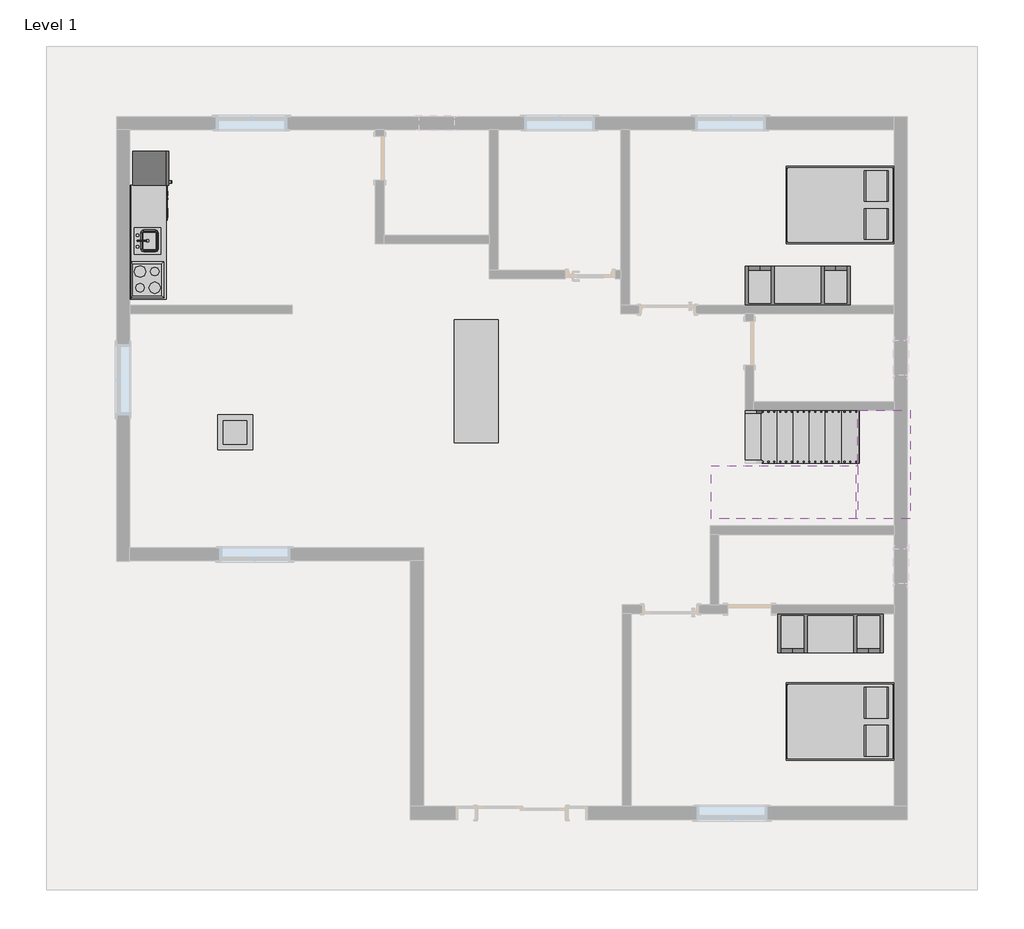
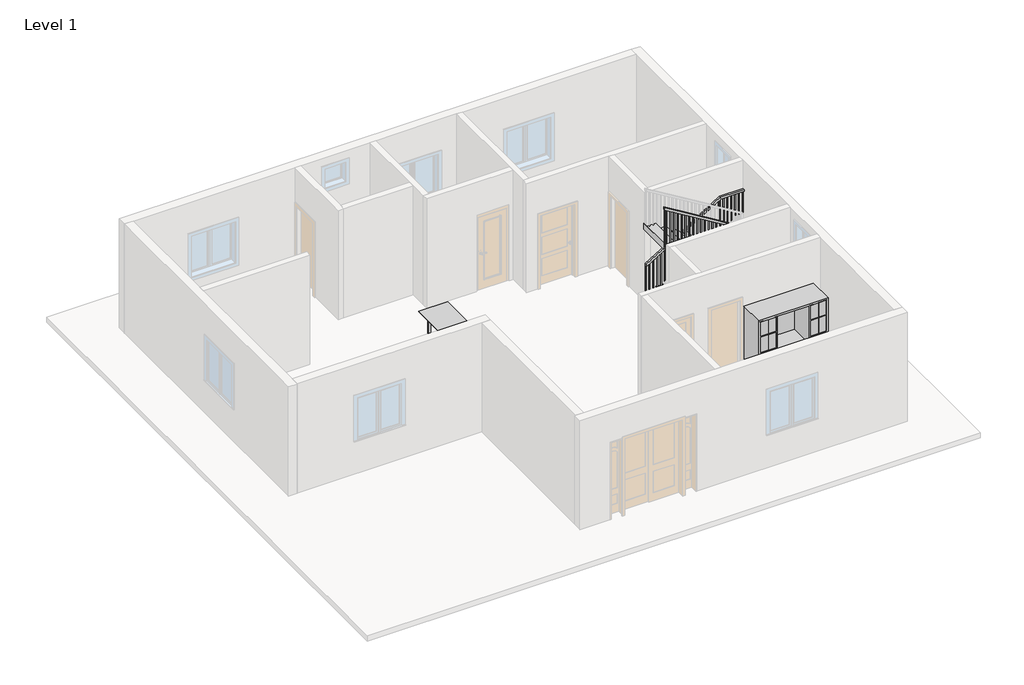
# One storey, part 2 of 2: 7 furniture elements, 4 proxies, 2 stair flights, 1 flow terminal, 1 railing, 1 slab.
"""IFC4 building model written with IfcOpenShell, lengths in millimetres."""

from ifc_helpers import new_model, si_unit, frame, origin, place, context, project, spatial, polyline, outline, extrude, faceted_brep, transform, mapped, element, save
from components import proxy_a6faaae8, proxy_45b28599, kitchenette_medium_0001_kitchenette_medium_0001_844211aa, proxy_c523a7b7, flow_terminal_871c2e40, furniture_c8abb964, furniture_c6510c7c, furniture_cf0b6580, furniture_b5c51a22, furniture_92191dda, non_monolithic_landing_284a18c3, stair_flight_c73b5a8b, stair_flight_e67f926d

model = new_model("IFC4")

# Units and contexts
model_context = context("Model", 3, world=origin())
ifc_project = project(units=[si_unit("LENGTHUNIT", "METRE", prefix="MILLI")], contexts=[model_context])

# Site, building, storey
site = spatial("IfcSite", under=ifc_project)
building = spatial("IfcBuilding", under=site)
storey = spatial("IfcBuildingStorey", under=building, Name="Level 1", Elevation=0.0)

# Proxies
placement = place(None, origin())
proxy_shape = proxy_a6faaae8(model_context)
element("IfcBuildingElementProxy", 1, Name="Cook Top-4 Unit2 : 22\" x 20\"", ObjectType="Cook Top-4 Unit2 : 22\" x 20\"", at=placement, inside=storey, context=model_context, shape_type="MappedRepresentation", body=[
    mapped(proxy_shape, transform((-14025.3866603, -262.6331121, 0.0), x_axis=(0.0, 1.0000000000000002, 0.0), y_axis=(-1.0000000000000002, 0.0, 0.0), z_axis=(0.0, 0.0, 1.0))),
])
proxy_2_shape = proxy_45b28599(model_context)
element("IfcBuildingElementProxy", 2, Name="Dishwasher : 24\" x 24\" x 34\"", ObjectType="Dishwasher : 24\" x 24\" x 34\"", at=placement, inside=storey, context=model_context, shape_type="MappedRepresentation", body=[
    mapped(proxy_2_shape, transform((-13733.5370955, 688.5494195, 0.0), x_axis=(0.0, 1.0000000000000002, 0.0), y_axis=(-1.0000000000000002, 0.0, 0.0), z_axis=(0.0, 0.0, 1.0))),
])
kitchenette_medium_0001_kitchenette_medium_0001_shape = kitchenette_medium_0001_kitchenette_medium_0001_844211aa(model_context)
element("IfcBuildingElementProxy", 3, Name="Kitchenette - Medium.0001 : Kitchenette - Medium.0001", ObjectType="Kitchenette - Medium.0001 : Kitchenette - Medium.0001", at=placement, inside=storey, context=model_context, shape_type="MappedRepresentation", body=[
    mapped(kitchenette_medium_0001_kitchenette_medium_0001_shape, transform((-14330.1866603, 61.529183, 0.0), x_axis=(0.0, 1.0000000000000002, 0.0), y_axis=(-1.0000000000000002, 0.0, 0.0), z_axis=(0.0, 0.0, 1.0))),
])
proxy_3_shape = proxy_c523a7b7(model_context)
element("IfcBuildingElementProxy", 4, Name="Refrigerator : 24\" x 25\" LH", ObjectType="Refrigerator : 24\" x 25\" LH", at=placement, inside=storey, context=model_context, shape_type="MappedRepresentation", body=[
    mapped(proxy_3_shape, transform((-13979.7376888, 1674.1168879, 0.0), x_axis=(0.0, 1.0000000000000002, 0.0), y_axis=(-1.0000000000000002, 0.0, 0.0), z_axis=(0.0, 0.0, 1.0))),
])

# Flow terminal
flow_terminal_shape = flow_terminal_871c2e40(model_context)
element("IfcFlowTerminal", 5, ObjectType="Sink Kitchen-Island : 18\" x 18\"", at=placement, inside=storey, context=model_context, shape_type="MappedRepresentation", body=[
    mapped(flow_terminal_shape, transform((-14023.0412592, 394.7776474, -14.4), x_axis=(0.0, 1.0000000000000002, 0.0), y_axis=(-1.0000000000000002, 0.0, 0.0), z_axis=(0.0, 0.0, 1.0))),
])

# Furniture
furniture_shape = furniture_c8abb964(model_context)
element("IfcFurniture", 6, ObjectType="Bed-Box : Double 53\" x 74\"", at=placement, inside=storey, context=model_context, shape_type="MappedRepresentation", body=[
    mapped(furniture_shape, transform((-1751.3571521, 1371.919347, 0.0), x_axis=(0.0, -0.9999999999999998, 0.0), y_axis=(0.9999999999999998, 0.0, 0.0), z_axis=(0.0, 0.0, 1.0))),
])
element("IfcFurniture", 7, ObjectType="Bed-Box : Double 53\" x 74\"", at=placement, inside=storey, context=model_context, shape_type="MappedRepresentation", body=[
    mapped(furniture_shape, transform((-1751.3571521, -7606.980653, 0.0), x_axis=(0.0, -1.0, 0.0), y_axis=(1.0, 0.0, 0.0), z_axis=(0.0, 0.0, 1.0))),
])
furniture_2_shape = furniture_c6510c7c(model_context)
element("IfcFurniture", 8, ObjectType="Counter Top w Sink Hole : 24\" Depth", at=placement, inside=storey, context=model_context, shape_type="MappedRepresentation", body=[
    mapped(furniture_2_shape, transform((-14330.1866603, 594.929183, -14.4), x_axis=(0.0, 1.0000000000000002, 0.0), y_axis=(-1.0000000000000002, 0.0, 0.0), z_axis=(0.0, 0.0, 1.0))),
])
furniture_3_shape = furniture_cf0b6580(model_context)
element("IfcFurniture", 9, ObjectType="Entertainment Center : 72\" x 72\" x 24\"", at=placement, inside=storey, context=model_context, shape_type="MappedRepresentation", body=[
    mapped(furniture_3_shape, transform((-2722.3866603, -808.7331121, 0.0), x_axis=(-1.0, 0.0, 0.0), y_axis=(0.0, -1.0, 0.0), z_axis=(0.0, 0.0, 1.0))),
])
element("IfcFurniture", 10, ObjectType="Entertainment Center : 72\" x 72\" x 24\"", at=placement, inside=storey, context=model_context, shape_type="MappedRepresentation", body=[
    mapped(furniture_3_shape, transform((-2150.8866603, -5964.9331121, 0.0), x_axis=(1.0000000000000002, 0.0, 0.0), y_axis=(0.0, 1.0000000000000002, 0.0), z_axis=(0.0, 0.0, 1.0))),
])
furniture_4_shape = furniture_b5c51a22(model_context)
element("IfcFurniture", 11, ObjectType="Table-Coffee : 24\" x 24\" x 24\"", at=placement, inside=storey, context=model_context, shape_type="MappedRepresentation", body=[
    mapped(furniture_4_shape, transform((-12519.6524269, -3012.1441899, 0.0), x_axis=(1.0, 0.0, 0.0), y_axis=(0.0, 1.0, 0.0), z_axis=(0.0, 0.0, 1.0))),
])
furniture_5_shape = furniture_92191dda(model_context)
element("IfcFurniture", 12, ObjectType="Table-Dining : 30\" x 84\" x 22\"", at=placement, inside=storey, context=model_context, shape_type="MappedRepresentation", body=[
    mapped(furniture_5_shape, transform((-8215.1755825, -2046.1988787, 0.0), x_axis=(0.0, 1.0, 0.0), y_axis=(-1.0, 0.0, 0.0), z_axis=(0.0, 0.0, 1.0))),
])

# Railing
element("IfcRailing", 13, ObjectType="Handrail - Rectangular", at=placement, inside=storey, context=model_context, shape_type="SolidModel", body=[
    faceted_brep([(-3636.7866603, -2535.9331121, 1083.7333333), (-3636.7866603, -2535.9331121, 1024.3318731), (-3636.7866603, -2586.7331121, 1024.3318731), (-3636.7866603, -2586.7331121, 1083.7333333), (-1680.9866603, -2535.9331121, 2269.0666667), (-1666.7942508, -2535.9331121, 2218.2666667), (-1666.7942508, -2586.7331121, 2218.2666667), (-1680.9866603, -2586.7331121, 2269.0666667), (-766.5866603, -2535.9331121, 2269.0666667), (-766.5866603, -2535.9331121, 2218.2666667), (-817.3866603, -2586.7331121, 2218.2666667), (-817.3866603, -2586.7331121, 2269.0666667), (-766.5866603, -4415.5331121, 2269.0666667), (-766.5866603, -4415.5331121, 2218.2666667), (-817.3866603, -4364.7331121, 2218.2666667), (-817.3866603, -4364.7331121, 2269.0666667), (-1401.5866603, -4415.5331121, 2269.0666667), (-1415.7790697, -4415.5331121, 2218.2666667), (-1415.7790697, -4364.7331121, 2218.2666667), (-1401.5866603, -4364.7331121, 2269.0666667), (-4195.5866603, -4415.5331121, 3962.4), (-4195.5866603, -4364.7331121, 3962.4), (-4195.5866603, -4364.7331121, 3902.9985397), (-4195.5866603, -4415.5331121, 3902.9985397)], [[[0, 1, 2, 3]], [[1, 0, 4, 5]], [[2, 1, 5, 6]], [[3, 2, 6, 7]], [[0, 3, 7, 4]], [[5, 4, 8, 9]], [[6, 5, 9, 10]], [[7, 6, 10, 11]], [[4, 7, 11, 8]], [[9, 8, 12, 13]], [[10, 9, 13, 14]], [[11, 10, 14, 15]], [[8, 11, 15, 12]], [[13, 12, 16, 17]], [[14, 13, 17, 18]], [[15, 14, 18, 19]], [[12, 15, 19, 16]], [[20, 21, 22, 23]], [[17, 16, 20, 23]], [[18, 17, 23, 22]], [[19, 18, 22, 21]], [[16, 19, 21, 20]]]),
    extrude(outline(polyline([(3877.9833882, -4154.3116603), (2878.6666667, -4154.3116603), (2878.6666667, -4135.2616603), (3866.4379337, -4135.2616603), (3877.9833882, -4154.3116603)])), frame((0.0, -4399.6581121, 0.0), z_axis=(0.0, 1.0, 0.0), x_axis=(0.0, 0.0, 1.0)), (0.0, 0.0, 1.0), 19.05),
    extrude(outline(polyline([(3816.4076307, -4052.7116603), (2878.6666667, -4052.7116603), (2878.6666667, -4033.6616603), (3804.8621761, -4033.6616603), (3816.4076307, -4052.7116603)])), frame((0.0, -4399.6581121, 0.0), z_axis=(0.0, 1.0, 0.0), x_axis=(0.0, 0.0, 1.0)), (0.0, 0.0, 1.0), 19.05),
    extrude(outline(polyline([(3754.8318731, -3951.1116603), (2878.6666667, -3951.1116603), (2878.6666667, -3932.0616603), (3743.2864185, -3932.0616603), (3754.8318731, -3951.1116603)])), frame((0.0, -4399.6581121, 0.0), z_axis=(0.0, 1.0, 0.0), x_axis=(0.0, 0.0, 1.0)), (0.0, 0.0, 1.0), 19.05),
    extrude(outline(polyline([(3693.2561155, -3849.5116603), (2709.3333333, -3849.5116603), (2709.3333333, -3830.4616603), (3681.710661, -3830.4616603), (3693.2561155, -3849.5116603)])), frame((0.0, -4399.6581121, 0.0), z_axis=(0.0, 1.0, 0.0), x_axis=(0.0, 0.0, 1.0)), (0.0, 0.0, 1.0), 19.05),
    extrude(outline(polyline([(3631.6803579, -3747.9116603), (2709.3333333, -3747.9116603), (2709.3333333, -3728.8616603), (3620.1349034, -3728.8616603), (3631.6803579, -3747.9116603)])), frame((0.0, -4399.6581121, 0.0), z_axis=(0.0, 1.0, 0.0), x_axis=(0.0, 0.0, 1.0)), (0.0, 0.0, 1.0), 19.05),
    extrude(outline(polyline([(3570.1046004, -3646.3116603), (2709.3333333, -3646.3116603), (2709.3333333, -3627.2616603), (3558.5591458, -3627.2616603), (3570.1046004, -3646.3116603)])), frame((0.0, -4399.6581121, 0.0), z_axis=(0.0, 1.0, 0.0), x_axis=(0.0, 0.0, 1.0)), (0.0, 0.0, 1.0), 19.05),
    extrude(outline(polyline([(3508.5288428, -3544.7116603), (2540.0, -3544.7116603), (2540.0, -3525.6616603), (3496.9833882, -3525.6616603), (3508.5288428, -3544.7116603)])), frame((0.0, -4399.6581121, 0.0), z_axis=(0.0, 1.0, 0.0), x_axis=(0.0, 0.0, 1.0)), (0.0, 0.0, 1.0), 19.05),
    extrude(outline(polyline([(3446.9530852, -3443.1116603), (2540.0, -3443.1116603), (2540.0, -3424.0616603), (3435.4076307, -3424.0616603), (3446.9530852, -3443.1116603)])), frame((0.0, -4399.6581121, 0.0), z_axis=(0.0, 1.0, 0.0), x_axis=(0.0, 0.0, 1.0)), (0.0, 0.0, 1.0), 19.05),
    extrude(outline(polyline([(3385.3773276, -3341.5116603), (2370.6666667, -3341.5116603), (2370.6666667, -3322.4616603), (3373.8318731, -3322.4616603), (3385.3773276, -3341.5116603)])), frame((0.0, -4399.6581121, 0.0), z_axis=(0.0, 1.0, 0.0), x_axis=(0.0, 0.0, 1.0)), (0.0, 0.0, 1.0), 19.05),
    extrude(outline(polyline([(3323.80157, -3239.9116603), (2370.6666667, -3239.9116603), (2370.6666667, -3220.8616603), (3312.2561155, -3220.8616603), (3323.80157, -3239.9116603)])), frame((0.0, -4399.6581121, 0.0), z_axis=(0.0, 1.0, 0.0), x_axis=(0.0, 0.0, 1.0)), (0.0, 0.0, 1.0), 19.05),
    extrude(outline(polyline([(3262.2258125, -3138.3116603), (2370.6666667, -3138.3116603), (2370.6666667, -3119.2616603), (3250.6803579, -3119.2616603), (3262.2258125, -3138.3116603)])), frame((0.0, -4399.6581121, 0.0), z_axis=(0.0, 1.0, 0.0), x_axis=(0.0, 0.0, 1.0)), (0.0, 0.0, 1.0), 19.05),
    extrude(outline(polyline([(3200.6500549, -3036.7116603), (2201.3333333, -3036.7116603), (2201.3333333, -3017.6616603), (3189.1046004, -3017.6616603), (3200.6500549, -3036.7116603)])), frame((0.0, -4399.6581121, 0.0), z_axis=(0.0, 1.0, 0.0), x_axis=(0.0, 0.0, 1.0)), (0.0, 0.0, 1.0), 19.05),
    extrude(outline(polyline([(3139.0742973, -2935.1116603), (2201.3333333, -2935.1116603), (2201.3333333, -2916.0616603), (3127.5288428, -2916.0616603), (3139.0742973, -2935.1116603)])), frame((0.0, -4399.6581121, 0.0), z_axis=(0.0, 1.0, 0.0), x_axis=(0.0, 0.0, 1.0)), (0.0, 0.0, 1.0), 19.05),
    extrude(outline(polyline([(3077.4985397, -2833.5116603), (2201.3333333, -2833.5116603), (2201.3333333, -2814.4616603), (3065.9530852, -2814.4616603), (3077.4985397, -2833.5116603)])), frame((0.0, -4399.6581121, 0.0), z_axis=(0.0, 1.0, 0.0), x_axis=(0.0, 0.0, 1.0)), (0.0, 0.0, 1.0), 19.05),
    extrude(outline(polyline([(3015.9227822, -2731.9116603), (2032.0, -2731.9116603), (2032.0, -2712.8616603), (3004.3773276, -2712.8616603), (3015.9227822, -2731.9116603)])), frame((0.0, -4399.6581121, 0.0), z_axis=(0.0, 1.0, 0.0), x_axis=(0.0, 0.0, 1.0)), (0.0, 0.0, 1.0), 19.05),
    extrude(outline(polyline([(2954.3470246, -2630.3116603), (2032.0, -2630.3116603), (2032.0, -2611.2616603), (2942.80157, -2611.2616603), (2954.3470246, -2630.3116603)])), frame((0.0, -4399.6581121, 0.0), z_axis=(0.0, 1.0, 0.0), x_axis=(0.0, 0.0, 1.0)), (0.0, 0.0, 1.0), 19.05),
    extrude(outline(polyline([(2892.771267, -2528.7116603), (2032.0, -2528.7116603), (2032.0, -2509.6616603), (2881.2258125, -2509.6616603), (2892.771267, -2528.7116603)])), frame((0.0, -4399.6581121, 0.0), z_axis=(0.0, 1.0, 0.0), x_axis=(0.0, 0.0, 1.0)), (0.0, 0.0, 1.0), 19.05),
    extrude(outline(polyline([(2831.1955094, -2427.1116603), (1862.6666667, -2427.1116603), (1862.6666667, -2408.0616603), (2819.6500549, -2408.0616603), (2831.1955094, -2427.1116603)])), frame((0.0, -4399.6581121, 0.0), z_axis=(0.0, 1.0, 0.0), x_axis=(0.0, 0.0, 1.0)), (0.0, 0.0, 1.0), 19.05),
    extrude(outline(polyline([(2769.6197519, -2325.5116603), (1862.6666667, -2325.5116603), (1862.6666667, -2306.4616603), (2758.0742973, -2306.4616603), (2769.6197519, -2325.5116603)])), frame((0.0, -4399.6581121, 0.0), z_axis=(0.0, 1.0, 0.0), x_axis=(0.0, 0.0, 1.0)), (0.0, 0.0, 1.0), 19.05),
    extrude(outline(polyline([(2708.0439943, -2223.9116603), (1693.3333333, -2223.9116603), (1693.3333333, -2204.8616603), (2696.4985397, -2204.8616603), (2708.0439943, -2223.9116603)])), frame((0.0, -4399.6581121, 0.0), z_axis=(0.0, 1.0, 0.0), x_axis=(0.0, 0.0, 1.0)), (0.0, 0.0, 1.0), 19.05),
    extrude(outline(polyline([(2646.4682367, -2122.3116603), (1693.3333333, -2122.3116603), (1693.3333333, -2103.2616603), (2634.9227822, -2103.2616603), (2646.4682367, -2122.3116603)])), frame((0.0, -4399.6581121, 0.0), z_axis=(0.0, 1.0, 0.0), x_axis=(0.0, 0.0, 1.0)), (0.0, 0.0, 1.0), 19.05),
    extrude(outline(polyline([(2584.8924791, -2020.7116603), (1693.3333333, -2020.7116603), (1693.3333333, -2001.6616603), (2573.3470246, -2001.6616603), (2584.8924791, -2020.7116603)])), frame((0.0, -4399.6581121, 0.0), z_axis=(0.0, 1.0, 0.0), x_axis=(0.0, 0.0, 1.0)), (0.0, 0.0, 1.0), 19.05),
    extrude(outline(polyline([(2523.3167216, -1919.1116603), (1524.0, -1919.1116603), (1524.0, -1900.0616603), (2511.771267, -1900.0616603), (2523.3167216, -1919.1116603)])), frame((0.0, -4399.6581121, 0.0), z_axis=(0.0, 1.0, 0.0), x_axis=(0.0, 0.0, 1.0)), (0.0, 0.0, 1.0), 19.05),
    extrude(outline(polyline([(2461.740964, -1817.5116603), (1524.0, -1817.5116603), (1524.0, -1798.4616603), (2450.1955094, -1798.4616603), (2461.740964, -1817.5116603)])), frame((0.0, -4399.6581121, 0.0), z_axis=(0.0, 1.0, 0.0), x_axis=(0.0, 0.0, 1.0)), (0.0, 0.0, 1.0), 19.05),
    extrude(outline(polyline([(2400.1652064, -1715.9116603), (1524.0, -1715.9116603), (1524.0, -1696.8616603), (2388.6197519, -1696.8616603), (2400.1652064, -1715.9116603)])), frame((0.0, -4399.6581121, 0.0), z_axis=(0.0, 1.0, 0.0), x_axis=(0.0, 0.0, 1.0)), (0.0, 0.0, 1.0), 19.05),
    extrude(outline(polyline([(2338.5894488, -1614.3116603), (1354.6666667, -1614.3116603), (1354.6666667, -1595.2616603), (2327.0439943, -1595.2616603), (2338.5894488, -1614.3116603)])), frame((0.0, -4399.6581121, 0.0), z_axis=(0.0, 1.0, 0.0), x_axis=(0.0, 0.0, 1.0)), (0.0, 0.0, 1.0), 19.05),
    extrude(outline(polyline([(2277.0136913, -1512.7116603), (1354.6666667, -1512.7116603), (1354.6666667, -1493.6616603), (2265.4682367, -1493.6616603), (2277.0136913, -1512.7116603)])), frame((0.0, -4399.6581121, 0.0), z_axis=(0.0, 1.0, 0.0), x_axis=(0.0, 0.0, 1.0)), (0.0, 0.0, 1.0), 19.05),
    extrude(outline(polyline([(-1290.4616603, -4399.6581121), (-1309.5116603, -4399.6581121), (-1309.5116603, -4380.6081121), (-1290.4616603, -4380.6081121), (-1290.4616603, -4399.6581121)])), frame((0.0, 0.0, 1354.6666667), z_axis=(0.0, 0.0, 1.0), x_axis=(1.0, 0.0, 0.0)), (0.0, 0.0, 1.0), 863.6),
    extrude(outline(polyline([(-1188.8616603, -4399.6581121), (-1207.9116603, -4399.6581121), (-1207.9116603, -4380.6081121), (-1188.8616603, -4380.6081121), (-1188.8616603, -4399.6581121)])), frame((0.0, 0.0, 1354.6666667), z_axis=(0.0, 0.0, 1.0), x_axis=(1.0, 0.0, 0.0)), (0.0, 0.0, 1.0), 863.6),
    extrude(outline(polyline([(-1087.2616603, -4399.6581121), (-1106.3116603, -4399.6581121), (-1106.3116603, -4380.6081121), (-1087.2616603, -4380.6081121), (-1087.2616603, -4399.6581121)])), frame((0.0, 0.0, 1354.6666667), z_axis=(0.0, 0.0, 1.0), x_axis=(1.0, 0.0, 0.0)), (0.0, 0.0, 1.0), 863.6),
    extrude(outline(polyline([(-985.6616603, -4399.6581121), (-1004.7116603, -4399.6581121), (-1004.7116603, -4380.6081121), (-985.6616603, -4380.6081121), (-985.6616603, -4399.6581121)])), frame((0.0, 0.0, 1354.6666667), z_axis=(0.0, 0.0, 1.0), x_axis=(1.0, 0.0, 0.0)), (0.0, 0.0, 1.0), 863.6),
    extrude(outline(polyline([(-884.0616603, -4399.6581121), (-903.1116603, -4399.6581121), (-903.1116603, -4380.6081121), (-884.0616603, -4380.6081121), (-884.0616603, -4399.6581121)])), frame((0.0, 0.0, 1354.6666667), z_axis=(0.0, 0.0, 1.0), x_axis=(1.0, 0.0, 0.0)), (0.0, 0.0, 1.0), 863.6),
    extrude(outline(polyline([(-782.4616603, -4279.0081121), (-782.4616603, -4298.0581121), (-801.5116603, -4298.0581121), (-801.5116603, -4279.0081121), (-782.4616603, -4279.0081121)])), frame((0.0, 0.0, 1354.6666667), z_axis=(0.0, 0.0, 1.0), x_axis=(1.0, 0.0, 0.0)), (0.0, 0.0, 1.0), 863.6),
    extrude(outline(polyline([(-782.4616603, -4177.4081121), (-782.4616603, -4196.4581121), (-801.5116603, -4196.4581121), (-801.5116603, -4177.4081121), (-782.4616603, -4177.4081121)])), frame((0.0, 0.0, 1354.6666667), z_axis=(0.0, 0.0, 1.0), x_axis=(1.0, 0.0, 0.0)), (0.0, 0.0, 1.0), 863.6),
    extrude(outline(polyline([(-782.4616603, -4075.8081121), (-782.4616603, -4094.8581121), (-801.5116603, -4094.8581121), (-801.5116603, -4075.8081121), (-782.4616603, -4075.8081121)])), frame((0.0, 0.0, 1354.6666667), z_axis=(0.0, 0.0, 1.0), x_axis=(1.0, 0.0, 0.0)), (0.0, 0.0, 1.0), 863.6),
    extrude(outline(polyline([(-782.4616603, -3974.2081121), (-782.4616603, -3993.2581121), (-801.5116603, -3993.2581121), (-801.5116603, -3974.2081121), (-782.4616603, -3974.2081121)])), frame((0.0, 0.0, 1354.6666667), z_axis=(0.0, 0.0, 1.0), x_axis=(1.0, 0.0, 0.0)), (0.0, 0.0, 1.0), 863.6),
    extrude(outline(polyline([(-782.4616603, -3872.6081121), (-782.4616603, -3891.6581121), (-801.5116603, -3891.6581121), (-801.5116603, -3872.6081121), (-782.4616603, -3872.6081121)])), frame((0.0, 0.0, 1354.6666667), z_axis=(0.0, 0.0, 1.0), x_axis=(1.0, 0.0, 0.0)), (0.0, 0.0, 1.0), 863.6),
    extrude(outline(polyline([(-782.4616603, -3771.0081121), (-782.4616603, -3790.0581121), (-801.5116603, -3790.0581121), (-801.5116603, -3771.0081121), (-782.4616603, -3771.0081121)])), frame((0.0, 0.0, 1354.6666667), z_axis=(0.0, 0.0, 1.0), x_axis=(1.0, 0.0, 0.0)), (0.0, 0.0, 1.0), 863.6),
    extrude(outline(polyline([(-782.4616603, -3669.4081121), (-782.4616603, -3688.4581121), (-801.5116603, -3688.4581121), (-801.5116603, -3669.4081121), (-782.4616603, -3669.4081121)])), frame((0.0, 0.0, 1354.6666667), z_axis=(0.0, 0.0, 1.0), x_axis=(1.0, 0.0, 0.0)), (0.0, 0.0, 1.0), 863.6),
    extrude(outline(polyline([(-782.4616603, -3567.8081121), (-782.4616603, -3586.8581121), (-801.5116603, -3586.8581121), (-801.5116603, -3567.8081121), (-782.4616603, -3567.8081121)])), frame((0.0, 0.0, 1354.6666667), z_axis=(0.0, 0.0, 1.0), x_axis=(1.0, 0.0, 0.0)), (0.0, 0.0, 1.0), 863.6),
    extrude(outline(polyline([(-782.4616603, -3466.2081121), (-782.4616603, -3485.2581121), (-801.5116603, -3485.2581121), (-801.5116603, -3466.2081121), (-782.4616603, -3466.2081121)])), frame((0.0, 0.0, 1354.6666667), z_axis=(0.0, 0.0, 1.0), x_axis=(1.0, 0.0, 0.0)), (0.0, 0.0, 1.0), 863.6),
    extrude(outline(polyline([(-782.4616603, -3364.6081121), (-782.4616603, -3383.6581121), (-801.5116603, -3383.6581121), (-801.5116603, -3364.6081121), (-782.4616603, -3364.6081121)])), frame((0.0, 0.0, 1354.6666667), z_axis=(0.0, 0.0, 1.0), x_axis=(1.0, 0.0, 0.0)), (0.0, 0.0, 1.0), 863.6),
    extrude(outline(polyline([(-782.4616603, -3263.0081121), (-782.4616603, -3282.0581121), (-801.5116603, -3282.0581121), (-801.5116603, -3263.0081121), (-782.4616603, -3263.0081121)])), frame((0.0, 0.0, 1354.6666667), z_axis=(0.0, 0.0, 1.0), x_axis=(1.0, 0.0, 0.0)), (0.0, 0.0, 1.0), 863.6),
    extrude(outline(polyline([(-782.4616603, -3161.4081121), (-782.4616603, -3180.4581121), (-801.5116603, -3180.4581121), (-801.5116603, -3161.4081121), (-782.4616603, -3161.4081121)])), frame((0.0, 0.0, 1354.6666667), z_axis=(0.0, 0.0, 1.0), x_axis=(1.0, 0.0, 0.0)), (0.0, 0.0, 1.0), 863.6),
    extrude(outline(polyline([(-782.4616603, -3059.8081121), (-782.4616603, -3078.8581121), (-801.5116603, -3078.8581121), (-801.5116603, -3059.8081121), (-782.4616603, -3059.8081121)])), frame((0.0, 0.0, 1354.6666667), z_axis=(0.0, 0.0, 1.0), x_axis=(1.0, 0.0, 0.0)), (0.0, 0.0, 1.0), 863.6),
    extrude(outline(polyline([(-782.4616603, -2958.2081121), (-782.4616603, -2977.2581121), (-801.5116603, -2977.2581121), (-801.5116603, -2958.2081121), (-782.4616603, -2958.2081121)])), frame((0.0, 0.0, 1354.6666667), z_axis=(0.0, 0.0, 1.0), x_axis=(1.0, 0.0, 0.0)), (0.0, 0.0, 1.0), 863.6),
    extrude(outline(polyline([(-782.4616603, -2856.6081121), (-782.4616603, -2875.6581121), (-801.5116603, -2875.6581121), (-801.5116603, -2856.6081121), (-782.4616603, -2856.6081121)])), frame((0.0, 0.0, 1354.6666667), z_axis=(0.0, 0.0, 1.0), x_axis=(1.0, 0.0, 0.0)), (0.0, 0.0, 1.0), 863.6),
    extrude(outline(polyline([(-782.4616603, -2755.0081121), (-782.4616603, -2774.0581121), (-801.5116603, -2774.0581121), (-801.5116603, -2755.0081121), (-782.4616603, -2755.0081121)])), frame((0.0, 0.0, 1354.6666667), z_axis=(0.0, 0.0, 1.0), x_axis=(1.0, 0.0, 0.0)), (0.0, 0.0, 1.0), 863.6),
    extrude(outline(polyline([(-782.4616603, -2653.4081121), (-782.4616603, -2672.4581121), (-801.5116603, -2672.4581121), (-801.5116603, -2653.4081121), (-782.4616603, -2653.4081121)])), frame((0.0, 0.0, 1354.6666667), z_axis=(0.0, 0.0, 1.0), x_axis=(1.0, 0.0, 0.0)), (0.0, 0.0, 1.0), 863.6),
    extrude(outline(polyline([(-877.7116603, -2551.8081121), (-858.6616603, -2551.8081121), (-858.6616603, -2570.8581121), (-877.7116603, -2570.8581121), (-877.7116603, -2551.8081121)])), frame((0.0, 0.0, 1354.6666667), z_axis=(0.0, 0.0, 1.0), x_axis=(1.0, 0.0, 0.0)), (0.0, 0.0, 1.0), 863.6),
    extrude(outline(polyline([(-979.3116603, -2551.8081121), (-960.2616603, -2551.8081121), (-960.2616603, -2570.8581121), (-979.3116603, -2570.8581121), (-979.3116603, -2551.8081121)])), frame((0.0, 0.0, 1354.6666667), z_axis=(0.0, 0.0, 1.0), x_axis=(1.0, 0.0, 0.0)), (0.0, 0.0, 1.0), 863.6),
    extrude(outline(polyline([(-1080.9116603, -2551.8081121), (-1061.8616603, -2551.8081121), (-1061.8616603, -2570.8581121), (-1080.9116603, -2570.8581121), (-1080.9116603, -2551.8081121)])), frame((0.0, 0.0, 1354.6666667), z_axis=(0.0, 0.0, 1.0), x_axis=(1.0, 0.0, 0.0)), (0.0, 0.0, 1.0), 863.6),
    extrude(outline(polyline([(-1182.5116603, -2551.8081121), (-1163.4616603, -2551.8081121), (-1163.4616603, -2570.8581121), (-1182.5116603, -2570.8581121), (-1182.5116603, -2551.8081121)])), frame((0.0, 0.0, 1354.6666667), z_axis=(0.0, 0.0, 1.0), x_axis=(1.0, 0.0, 0.0)), (0.0, 0.0, 1.0), 863.6),
    extrude(outline(polyline([(-1284.1116603, -2551.8081121), (-1265.0616603, -2551.8081121), (-1265.0616603, -2570.8581121), (-1284.1116603, -2570.8581121), (-1284.1116603, -2551.8081121)])), frame((0.0, 0.0, 1354.6666667), z_axis=(0.0, 0.0, 1.0), x_axis=(1.0, 0.0, 0.0)), (0.0, 0.0, 1.0), 863.6),
    extrude(outline(polyline([(-1385.7116603, -2551.8081121), (-1366.6616603, -2551.8081121), (-1366.6616603, -2570.8581121), (-1385.7116603, -2570.8581121), (-1385.7116603, -2551.8081121)])), frame((0.0, 0.0, 1354.6666667), z_axis=(0.0, 0.0, 1.0), x_axis=(1.0, 0.0, 0.0)), (0.0, 0.0, 1.0), 863.6),
    extrude(outline(polyline([(-1487.3116603, -2551.8081121), (-1468.2616603, -2551.8081121), (-1468.2616603, -2570.8581121), (-1487.3116603, -2570.8581121), (-1487.3116603, -2551.8081121)])), frame((0.0, 0.0, 1354.6666667), z_axis=(0.0, 0.0, 1.0), x_axis=(1.0, 0.0, 0.0)), (0.0, 0.0, 1.0), 863.6),
    extrude(outline(polyline([(-1588.9116603, -2551.8081121), (-1569.8616603, -2551.8081121), (-1569.8616603, -2570.8581121), (-1588.9116603, -2570.8581121), (-1588.9116603, -2551.8081121)])), frame((0.0, 0.0, 1354.6666667), z_axis=(0.0, 0.0, 1.0), x_axis=(1.0, 0.0, 0.0)), (0.0, 0.0, 1.0), 863.6),
    extrude(outline(polyline([(2188.4985397, -1715.9116603), (1185.3333333, -1715.9116603), (1185.3333333, -1696.8616603), (2200.0439943, -1696.8616603), (2188.4985397, -1715.9116603)])), frame((0.0, -2570.8581121, 0.0), z_axis=(0.0, 1.0, 0.0), x_axis=(0.0, 0.0, 1.0)), (0.0, 0.0, 1.0), 19.05),
    extrude(outline(polyline([(2126.9227822, -1817.5116603), (1185.3333333, -1817.5116603), (1185.3333333, -1798.4616603), (2138.4682367, -1798.4616603), (2126.9227822, -1817.5116603)])), frame((0.0, -2570.8581121, 0.0), z_axis=(0.0, 1.0, 0.0), x_axis=(0.0, 0.0, 1.0)), (0.0, 0.0, 1.0), 19.05),
    extrude(outline(polyline([(2065.3470246, -1919.1116603), (1185.3333333, -1919.1116603), (1185.3333333, -1900.0616603), (2076.8924791, -1900.0616603), (2065.3470246, -1919.1116603)])), frame((0.0, -2570.8581121, 0.0), z_axis=(0.0, 1.0, 0.0), x_axis=(0.0, 0.0, 1.0)), (0.0, 0.0, 1.0), 19.05),
    extrude(outline(polyline([(2003.771267, -2020.7116603), (1016.0, -2020.7116603), (1016.0, -2001.6616603), (2015.3167216, -2001.6616603), (2003.771267, -2020.7116603)])), frame((0.0, -2570.8581121, 0.0), z_axis=(0.0, 1.0, 0.0), x_axis=(0.0, 0.0, 1.0)), (0.0, 0.0, 1.0), 19.05),
    extrude(outline(polyline([(1942.1955094, -2122.3116603), (1016.0, -2122.3116603), (1016.0, -2103.2616603), (1953.740964, -2103.2616603), (1942.1955094, -2122.3116603)])), frame((0.0, -2570.8581121, 0.0), z_axis=(0.0, 1.0, 0.0), x_axis=(0.0, 0.0, 1.0)), (0.0, 0.0, 1.0), 19.05),
    extrude(outline(polyline([(1880.6197519, -2223.9116603), (1016.0, -2223.9116603), (1016.0, -2204.8616603), (1892.1652064, -2204.8616603), (1880.6197519, -2223.9116603)])), frame((0.0, -2570.8581121, 0.0), z_axis=(0.0, 1.0, 0.0), x_axis=(0.0, 0.0, 1.0)), (0.0, 0.0, 1.0), 19.05),
    extrude(outline(polyline([(1819.0439943, -2325.5116603), (846.6666667, -2325.5116603), (846.6666667, -2306.4616603), (1830.5894488, -2306.4616603), (1819.0439943, -2325.5116603)])), frame((0.0, -2570.8581121, 0.0), z_axis=(0.0, 1.0, 0.0), x_axis=(0.0, 0.0, 1.0)), (0.0, 0.0, 1.0), 19.05),
    extrude(outline(polyline([(1757.4682367, -2427.1116603), (846.6666667, -2427.1116603), (846.6666667, -2408.0616603), (1769.0136913, -2408.0616603), (1757.4682367, -2427.1116603)])), frame((0.0, -2570.8581121, 0.0), z_axis=(0.0, 1.0, 0.0), x_axis=(0.0, 0.0, 1.0)), (0.0, 0.0, 1.0), 19.05),
    extrude(outline(polyline([(1695.8924791, -2528.7116603), (846.6666667, -2528.7116603), (846.6666667, -2509.6616603), (1707.4379337, -2509.6616603), (1695.8924791, -2528.7116603)])), frame((0.0, -2570.8581121, 0.0), z_axis=(0.0, 1.0, 0.0), x_axis=(0.0, 0.0, 1.0)), (0.0, 0.0, 1.0), 19.05),
    extrude(outline(polyline([(1634.3167216, -2630.3116603), (677.3333333, -2630.3116603), (677.3333333, -2611.2616603), (1645.8621761, -2611.2616603), (1634.3167216, -2630.3116603)])), frame((0.0, -2570.8581121, 0.0), z_axis=(0.0, 1.0, 0.0), x_axis=(0.0, 0.0, 1.0)), (0.0, 0.0, 1.0), 19.05),
    extrude(outline(polyline([(1572.740964, -2731.9116603), (677.3333333, -2731.9116603), (677.3333333, -2712.8616603), (1584.2864185, -2712.8616603), (1572.740964, -2731.9116603)])), frame((0.0, -2570.8581121, 0.0), z_axis=(0.0, 1.0, 0.0), x_axis=(0.0, 0.0, 1.0)), (0.0, 0.0, 1.0), 19.05),
    extrude(outline(polyline([(1511.1652064, -2833.5116603), (508.0, -2833.5116603), (508.0, -2814.4616603), (1522.710661, -2814.4616603), (1511.1652064, -2833.5116603)])), frame((0.0, -2570.8581121, 0.0), z_axis=(0.0, 1.0, 0.0), x_axis=(0.0, 0.0, 1.0)), (0.0, 0.0, 1.0), 19.05),
    extrude(outline(polyline([(1449.5894488, -2935.1116603), (508.0, -2935.1116603), (508.0, -2916.0616603), (1461.1349034, -2916.0616603), (1449.5894488, -2935.1116603)])), frame((0.0, -2570.8581121, 0.0), z_axis=(0.0, 1.0, 0.0), x_axis=(0.0, 0.0, 1.0)), (0.0, 0.0, 1.0), 19.05),
    extrude(outline(polyline([(1388.0136913, -3036.7116603), (508.0, -3036.7116603), (508.0, -3017.6616603), (1399.5591458, -3017.6616603), (1388.0136913, -3036.7116603)])), frame((0.0, -2570.8581121, 0.0), z_axis=(0.0, 1.0, 0.0), x_axis=(0.0, 0.0, 1.0)), (0.0, 0.0, 1.0), 19.05),
    extrude(outline(polyline([(1326.4379337, -3138.3116603), (338.6666667, -3138.3116603), (338.6666667, -3119.2616603), (1337.9833882, -3119.2616603), (1326.4379337, -3138.3116603)])), frame((0.0, -2570.8581121, 0.0), z_axis=(0.0, 1.0, 0.0), x_axis=(0.0, 0.0, 1.0)), (0.0, 0.0, 1.0), 19.05),
    extrude(outline(polyline([(1264.8621761, -3239.9116603), (338.6666667, -3239.9116603), (338.6666667, -3220.8616603), (1276.4076307, -3220.8616603), (1264.8621761, -3239.9116603)])), frame((0.0, -2570.8581121, 0.0), z_axis=(0.0, 1.0, 0.0), x_axis=(0.0, 0.0, 1.0)), (0.0, 0.0, 1.0), 19.05),
    extrude(outline(polyline([(1203.2864185, -3341.5116603), (338.6666667, -3341.5116603), (338.6666667, -3322.4616603), (1214.8318731, -3322.4616603), (1203.2864185, -3341.5116603)])), frame((0.0, -2570.8581121, 0.0), z_axis=(0.0, 1.0, 0.0), x_axis=(0.0, 0.0, 1.0)), (0.0, 0.0, 1.0), 19.05),
    extrude(outline(polyline([(1141.710661, -3443.1116603), (169.3333333, -3443.1116603), (169.3333333, -3424.0616603), (1153.2561155, -3424.0616603), (1141.710661, -3443.1116603)])), frame((0.0, -2570.8581121, 0.0), z_axis=(0.0, 1.0, 0.0), x_axis=(0.0, 0.0, 1.0)), (0.0, 0.0, 1.0), 19.05),
    extrude(outline(polyline([(1080.1349034, -3544.7116603), (169.3333333, -3544.7116603), (169.3333333, -3525.6616603), (1091.6803579, -3525.6616603), (1080.1349034, -3544.7116603)])), frame((0.0, -2570.8581121, 0.0), z_axis=(0.0, 1.0, 0.0), x_axis=(0.0, 0.0, 1.0)), (0.0, 0.0, 1.0), 19.05),
    extrude(outline(polyline([(-1392.0616603, -4399.6581121), (-1411.1116603, -4399.6581121), (-1411.1116603, -4380.6081121), (-1392.0616603, -4380.6081121), (-1392.0616603, -4399.6581121)])), frame((0.0, 0.0, 1354.6666667), z_axis=(0.0, 0.0, 1.0), x_axis=(1.0, 0.0, 0.0)), (0.0, 0.0, 1.0), 863.6),
    extrude(outline(polyline([(-782.4616603, -4380.6081121), (-782.4616603, -4399.6581121), (-801.5116603, -4399.6581121), (-801.5116603, -4380.6081121), (-782.4616603, -4380.6081121)])), frame((0.0, 0.0, 1354.6666667), z_axis=(0.0, 0.0, 1.0), x_axis=(1.0, 0.0, 0.0)), (0.0, 0.0, 1.0), 863.6),
    extrude(outline(polyline([(-801.5116603, -2551.8081121), (-782.4616603, -2551.8081121), (-782.4616603, -2570.8581121), (-801.5116603, -2570.8581121), (-801.5116603, -2551.8081121)])), frame((0.0, 0.0, 1354.6666667), z_axis=(0.0, 0.0, 1.0), x_axis=(1.0, 0.0, 0.0)), (0.0, 0.0, 1.0), 863.6),
    extrude(outline(polyline([(-1690.5116603, -2551.8081121), (-1671.4616603, -2551.8081121), (-1671.4616603, -2570.8581121), (-1690.5116603, -2570.8581121), (-1690.5116603, -2551.8081121)])), frame((0.0, 0.0, 1354.6666667), z_axis=(0.0, 0.0, 1.0), x_axis=(1.0, 0.0, 0.0)), (0.0, 0.0, 1.0), 863.6),
    extrude(outline(polyline([(3902.9985397, -4195.5866603), (2878.6666667, -4195.5866603), (2878.6666667, -4176.5366603), (3891.4530852, -4176.5366603), (3902.9985397, -4195.5866603)])), frame((0.0, -4399.6581121, 0.0), z_axis=(0.0, 1.0, 0.0), x_axis=(0.0, 0.0, 1.0)), (0.0, 0.0, 1.0), 19.05),
    extrude(outline(polyline([(1024.3318731, -3636.7866603), (169.3333333, -3636.7866603), (169.3333333, -3617.7366603), (1035.8773276, -3617.7366603), (1024.3318731, -3636.7866603)])), frame((0.0, -2570.8581121, 0.0), z_axis=(0.0, 1.0, 0.0), x_axis=(0.0, 0.0, 1.0)), (0.0, 0.0, 1.0), 19.05),
])

# Slab
non_monolithic_landing_shape = non_monolithic_landing_284a18c3(model_context)
element("IfcSlab", 14, ObjectType="Non-Monolithic Landing", at=placement, inside=storey, context=model_context, shape_type="MappedRepresentation", body=[
    mapped(non_monolithic_landing_shape, transform((0.0, 0.0, 0.0), x_axis=(1.0, 0.0, 0.0), y_axis=(0.0, 1.0, 0.0), z_axis=(0.0, 0.0, 1.0))),
])

# Stair flights
stair_flight_shape = stair_flight_c73b5a8b(model_context)
element("IfcStairFlight", 15, ObjectType="2\" Tread 1\" Nosing 1/4\" Riser", at=placement, inside=storey, context=model_context, shape_type="MappedRepresentation", body=[
    mapped(stair_flight_shape, transform((0.0, 0.0, 0.0), x_axis=(1.0, 0.0, 0.0), y_axis=(0.0, 1.0, 0.0), z_axis=(0.0, 0.0, 1.0))),
])
stair_flight_2_shape = stair_flight_e67f926d(model_context)
element("IfcStairFlight", 16, ObjectType="2\" Tread 1\" Nosing 1/4\" Riser", at=placement, inside=storey, context=model_context, shape_type="MappedRepresentation", body=[
    mapped(stair_flight_2_shape, transform((0.0, 0.0, 0.0), x_axis=(1.0, 0.0, 0.0), y_axis=(0.0, 1.0, 0.0), z_axis=(0.0, 0.0, 1.0))),
])

save(model, "model.ifc")

# Revit data of these elements
# Type "Cook Top-4 Unit2 : 22\" x 20\""
#   Depth = 1' - 8"
#   Width = 1' - 10"
#   Burner Material = Steel, Chrome Plated
#   Cooktop Material = Steel, Polished
#   Default Elevation = 0
#   Assembly Code = ""
# Type "Dishwasher : 24\" x 24\" x 34\""
#   Label = "DW"
#   Assembly Code = "E1090400"
#   Depth = 2' - 0"
#   Height = 2' - 10"
#   Width = 2' - 0"
#   Dishwasher Material = Steel, Paint Finish, Ivory, Glossy
#   Panel Face Material = Plastic, Opaque Black
#   Default Elevation = 0
# Type "Kitchenette - Medium.0001 : Kitchenette - Medium.0001"
#   Assembly Code = "E1090400"
#   Counter Length = 6' - 6"
#   Cabinet Width = 4' - 6"
#   Cabinet Height = 2' - 10 1/2"
#   Cabinet Depth = 2' - 0"
#   Toe Depth = 0' - 3"
#   Toe Height = 0' - 3 1/2"
#   Cabinet Material = Cabinets
#   Door/Drawer Material = Cabinets
#   Handle Material = Cabinets - Handles
#   Default Elevation = 0
# Type "Refrigerator : 24\" x 25\" LH"
#   Label = "REF."
#   Assembly Code = "E1090400"
#   Depth = 2' - 0 3/4"
#   Handle = 0' - 1 1/2"
#   Height = 5' - 3 1/2"
#   Rear Clearance = 0' - 2"
#   Top Door Height = 1' - 8"
#   Width = 1' - 11 1/2"
#   Material = Steel, Paint Finish, Ivory, Glossy
#   Default Elevation = 0
# Type "Sink Kitchen-Island : 18\" x 18\""
#   Assembly Code = "D2010410"
#   Counter Height = 3' - 0"
#   Depth = 1' - 6"
#   Width = 1' - 6"
#   Faucet Material = Steel, Polished
#   Sink Material = Steel, Polished
#   Default Elevation = 0
# Type "Bed-Box : Double 53\" x 74\""
#   Assembly Code = "E2020200"
#   Length = 6' - 2"
#   Width = 4' - 5"
#   Frame Material = Birch
#   Mattress Material = Linen, White
#   Default Elevation = 0
# Type "Counter Top w Sink Hole : 24\" Depth"
#   Assembly Code = "C1030400"
#   Counter Thickness = 0' - 1 1/2"
#   Depth = 2' - 1"
#   Height = 3' - 0"
#   Length [instance default] = 8' - 0"
#   Sink Location [instance default] = 2' - 0"
#   Sink Location To Wall [instance default] = 0' - 6"
#   Sink Opening Depth [instance default] = 1' - 3"
#   Sink Opening Width [instance default] = 2' - 3"
#   Counter Top Material = none
#   Default Elevation = 0
# Type "Entertainment Center : 72\" x 72\" x 24\""
#   Assembly Code = "E2020200"
#   Center Width = 2' - 8"
#   Depth = 2' - 0"
#   Height = 6' - 0"
#   Width = 6' - 0"
#   Material = none
#   Default Elevation = 0
# Type "Table-Coffee : 24\" x 24\" x 24\""
#   Assembly Code = "E2020200"
#   Height = 2' - 0"
#   Length = 2' - 0"
#   Width = 2' - 0"
#   Top Material = none
#   Frame Material = none
#   Default Elevation = 0
# Type "Table-Dining : 30\" x 84\" x 22\""
#   Assembly Code = "E2020200"
#   Height = 1' - 10"
#   Length = 7' - 0"
#   Width = 2' - 6"
#   Base Material = Steel, Chrome Plated
#   Top Material = Glass - Clear, Grey
#   Default Elevation = 0
# Type "Handrail - Rectangular"
#   Assembly Code = "C2010400"
#   built-in parameter 1008612 = 0.0416667 (stored number, unit not read)
#   built-in parameter 1008611 = 0.0416667 (stored number, unit not read)
#   built-in parameter 1008609 = 0.333333 (stored number, unit not read)
#   built-in parameter 1008604 = 0.166667 (stored number, unit not read)
#   built-in parameter 1008603 = 0.166667 (stored number, unit not read)
#   Railing Height = 3' - 0"
#   built-in parameter 1008630 = 2
#   built-in parameter 1008610 = 2
#   built-in parameter 1008618 = Baluster - Square : 3/4"
# Element 1 (IfcBuildingElementProxy, "Cook Top-4 Unit2 : 22\" x 20\"")
#   Phase Created = New Construction
#   Materials on its faces: "Steel, Chrome Plated", "Steel, Polished"
# Element 2 (IfcBuildingElementProxy, "Dishwasher : 24\" x 24\" x 34\"")
#   Phase Created = New Construction
#   Materials on its faces: "Steel, Paint Finish, Ivory, Glossy", "Plastic, Opaque Black"
# Element 3 (IfcBuildingElementProxy, "Kitchenette - Medium.0001 : Kitchenette - Medium.0001")
#   Phase Created = New Construction
#   Materials on its faces: "Cabinets", "Cabinets - Handles"
# Element 4 (IfcBuildingElementProxy, "Refrigerator : 24\" x 25\" LH")
#   Phase Created = New Construction
#   Materials on its faces: "Steel, Paint Finish, Ivory, Glossy", "Steel, Chrome Plated"
# Element 5 (IfcFlowTerminal, "Sink Kitchen-Island : 18\" x 18\"")
#   Mark = "2"
#   Phase Created = New Construction
#   Materials on its faces: "Steel, Polished"
# Elements 6, 7 (IfcFurniture, "Bed-Box : Double 53\" x 74\"")
#   Phase Created = New Construction
#   Materials on its faces: "Birch", "Linen, White"
# Element 8 (IfcFurniture, "Counter Top w Sink Hole : 24\" Depth")
#   Sink Opening Depth = 1' - 2"
#   Sink Location To Wall = 0' - 6"
#   Length = 6' - 6"
#   Sink Location = 3' - 4"
#   Sink Opening Width = 1' - 4"
#   Phase Created = New Construction
#   Materials on its faces: "Counter Top"
# Elements 9, 10 (IfcFurniture, "Entertainment Center : 72\" x 72\" x 24\"")
#   Phase Created = New Construction
#   Materials on its faces: "Steel, Chrome Plated", "Glass - Clear, Grey"
# Element 11 (IfcFurniture, "Table-Coffee : 24\" x 24\" x 24\"")
#   Phase Created = New Construction
#   Materials on its faces: "Glass - Clear, Grey"
# Element 12 (IfcFurniture, "Table-Dining : 30\" x 84\" x 22\"")
#   Phase Created = New Construction
#   Materials on its faces: "Steel, Chrome Plated", "Glass - Clear, Grey"
# Element 13 (IfcRailing, "Handrail - Rectangular")
#   Phase Created = New Construction
# Element 14 (IfcSlab, "Non-Monolithic Landing")
#   Phase Created = New Construction
# Elements 15, 16 (IfcStairFlight, "2\" Tread 1\" Nosing 1/4\" Riser")
#   Phase Created = New Construction
# Materials
#   "Steel, Chrome Plated": class "Metal", colour RGB 17 17 17, transparency 0, Description = "Chromiuim plated steel", Cost = 0
#   "Steel, Polished": class "Metal", colour RGB 57 57 57, transparency 0, Description = "Polished steel", Cost = 0
#   "Steel, Paint Finish, Ivory, Glossy": class "Metal", colour RGB 247 247 239, transparency 0, Description = "Steel, paint finish, ivory, glossy", Cost = 0
#   "Plastic, Opaque Black": class "Plastic", colour RGB 0 0 0, transparency 0.7, Description = "Plastic, generic, opaque black", Cost = 0
#   "Cabinets": colour RGB 249 249 249, transparency 0
#   "Cabinets - Handles": class "Metal", colour RGB 57 57 57, transparency 0
#   "Birch": class "Wood", colour RGB 224 178 126, transparency 0, Description = "Betula Alleghaniensis", Cost = 0
#   "Linen, White": class "Textile", colour RGB 247 247 239, transparency 0, Description = "Linen, white", Cost = 0
#   "Glass - Clear, Grey": class "Glass", colour RGB 252 255 255, transparency 0.64
#   "Counter Top": class "Wood", colour RGB 226 177 128, transparency 0
